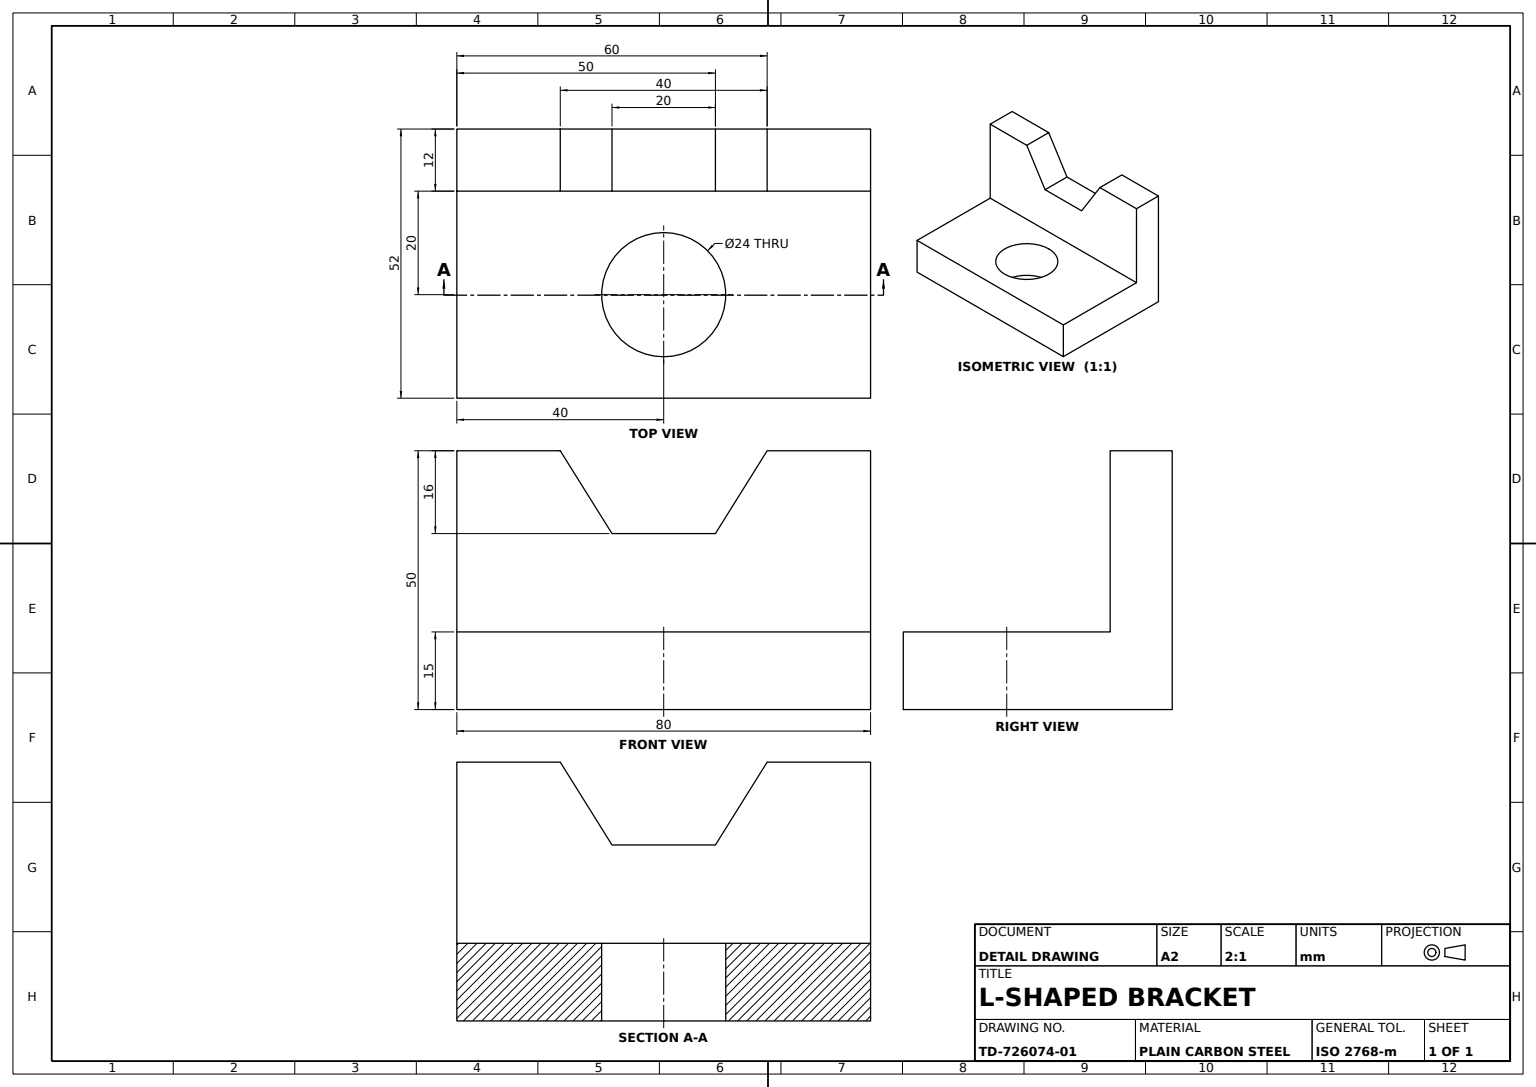
SolidWorks part; units mm, degrees
material "Plain Carbon Steel"
ref_plane "Front Plane" through (0, 0, 0) normal (0, 0, 1) x (1, 0, 0)
ref_plane "Top Plane" through (0, 0, 0) normal (0, 1, 0) x (1, 0, 0)
ref_plane "Right Plane" through (0, 0, 0) normal (1, 0, 0) x (0, 0, -1)
sketch "Upright V-Notch Profile Sketch" plane through (0, 0, 0) normal (0, 0, 1) x (1, 0, 0)
  line L0 (0, 0) -> (0, -50)
  line L1 (0, -50) -> (80, -50)
  line L2 (80, -50) -> (80, 0)
  line L3 (80, 0) -> (60, 0)
  line L6 (50, -16) -> (30, -16)
  line L7 (0, 0) -> (20, 0)
  line L8 (20, 0) -> (30, -16)
  line L9 (50, -16) -> (60, 0)
  dimension "D1" = 80
  dimension "D2" = 50
  dimension "D3" = 16
  dimension "D4" = 30
  dimension "D5" = 20
  dimension "D6" = 50
  dimension "D7" = 60
extrude "Upright V-Notch Plate" add sketch "Upright V-Notch Profile Sketch" along normal blind 12
sketch "Base Plate Sketch" plane through (0, 0, 12) normal (0, 0, 1) x (1, 0, 0)
  line L0 (80, -50) -> (80, 0) construction
  line L1 (0, -50) -> (80, -50)
  line L2 (0, -50) -> (0, -35)
  line L3 (0, -35) -> (80, -35)
  line L4 (80, -50) -> (80, -35)
  dimension "D1" = 15
extrude "Base Plate" add sketch "Base Plate Sketch" along normal blind 40
sketch "Base Hole Sketch Ø24" plane through (0, -35, 0) normal (0, 1, 0) x (1, 0, 0)
  line L0 (0, -52) -> (0, -12) construction
  line L1 (80, -12) -> (0, -12) construction
  circle A0 centre (40, -32) radius 12
  dimension "D1" = 24
  dimension "D2" = 24
  dimension "D3" = 40
  dimension "D4" = 20
extrude "Base Hole Ø24" cut sketch "Base Hole Sketch Ø24" against normal blind 20
